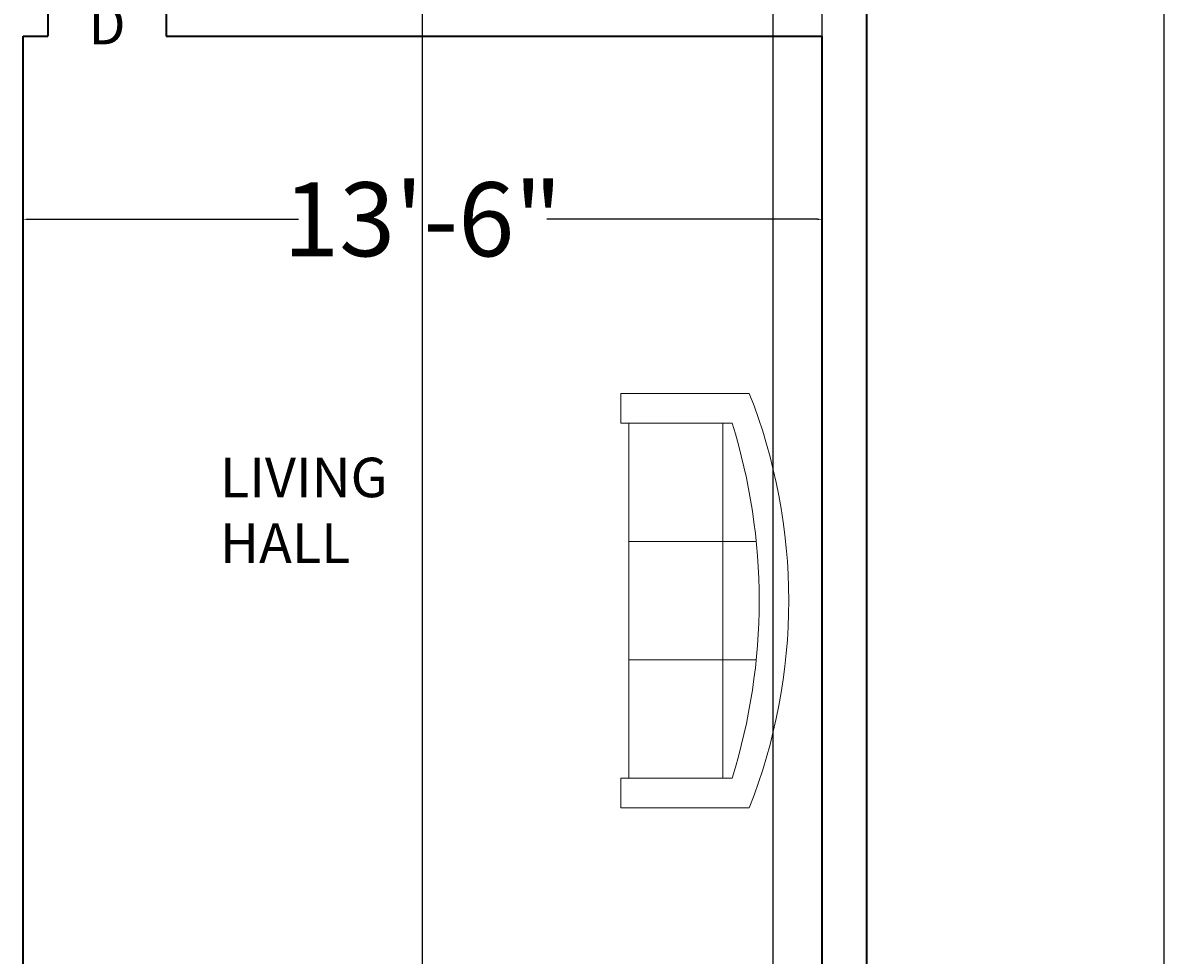
# Model space of a CAD drawing. Units: inches. Extents: x 371 to 1095, y -45 to 1219.
# Tile 13 of 18: x 862 to 1095, y 610 to 799. Entities that reach past the tile are written whole.
import ezdxf

# ---------------------------------------------------------------- set-up
doc = ezdxf.new("R2010")
doc.units = ezdxf.units.IN
doc.header["$MEASUREMENT"] = 0
for name, color, linetype, lineweight in [('A-ANNO-DIMS', 2, 'Continuous', 18), ('A-ANNO-TEXT', 7, 'Continuous', 18), ('A-AREA-IDEN', 7, 'Continuous', 18), ('A-FURN', 254, 'Continuous', 18), ('A-WALL', 40, 'Continuous', 35)]:
    doc.layers.add(name, color=color, linetype=linetype, lineweight=lineweight)
doc.styles.get("Standard").update_dxf_attribs({"font": 'arial.ttf'})
doc.dimstyles.get("Standard").update_dxf_attribs({"dimtxt": 1, "dimasz": 1, "dimexe": 0.18, "dimexo": 0.0625, "dimgap": 0.09, "dimtad": 0, "dimtih": 1, "dimtoh": 1, "dimdec": 0, "dimzin": 0, "dimdsep": 46, "dimlunit": 3, "dimtxsty": 'Standard', "dimcen": 0.09, "dimadec": 0, "dimazin": 0, "dimtfac": 1, "dimtdec": 0, "dimtofl": 0, "dimtmove": 0, "dimatfit": 3, "dimfxl": 1, "dimtolj": 1, "dimtzin": 0, "dimarcsym": 0})

# ---------------------------------------------------------------- blocks, each defined once
blk = doc.blocks.new('Sofa - Roundback 7 ft.')
for p, q in [((-12.00002, -32.4421), (-12.00003, -6.5971)), ((11.99997, -32.4421), (11.99998, -6.5971)), ((-36.000027, -34), (-36.000027, -11.4696)), ((35.99998, -34), (35.99998, -11.4696)), ((-35.999844, -13.3819), (35.9998, -13.3819)), ((-36.000027, -32.4421), (35.99998, -32.4421))]:
    blk.add_line(p, q)
for points in [[(-36.000027, -34), (-42.000027, -34), (-42.000027, -8)], [(41.99998, -8), (41.99998, -34), (35.99998, -34)]]:
    blk.add_lwpolyline(points)
for centre, radius, start, end in [((0, -114.25), 114.25, 68.43141, 111.5686), ((-0.00001, -127.1968), 121.1968, 72.72033, 107.2797)]:
    blk.add_arc(centre, radius, start, end)
blk = doc.blocks.new('*D24')
at = {"layer": 'A-ANNO-DIMS', "color": 0, "lineweight": -2, "transparency": 16777216}
for p, q in [((861.81, 748.67), (861.81, 759.09)), ((862.81, 758.91), (917.66, 758.91)), ((1022.81, 758.91), (967.96, 758.91)), ((1023.81, 748.67), (1023.81, 759.09))]:
    blk.add_line(p, q, dxfattribs=at)
at = {"layer": 'A-ANNO-DIMS', "color": 0, "transparency": 16777216}
for points in [[(862.81, 759.07), (862.81, 758.74), (861.81, 758.91)], [(1022.81, 759.07), (1022.81, 758.74), (1023.81, 758.91)]]:
    blk.add_solid(points, dxfattribs=at)
at = {"layer": 'Defpoints', "color": 0, "transparency": 16777216}
for p in [(1023.81, 758.91), (861.81, 748.61), (1023.81, 748.61)]:
    blk.add_point(p, dxfattribs=at)
at = {"layer": 'A-ANNO-DIMS', "color": 0, "transparency": 16777216, "insert": (942.81, 758.91), "char_height": 1, "attachment_point": 5}
blk.add_mtext('\\A1;{\\H15x;13\'-6"}', dxfattribs=at)
blk = doc.blocks.new('*D51')
at = {"layer": 'A-ANNO-DIMS', "color": 0, "lineweight": -2, "transparency": 16777216}
for p, q in [((1032.87, 982.03), (1093.19, 982.03)), ((1093.01, 981.03), (1093.01, 532.63)), ((1093.01, 83.03), (1093.01, 531.42)), ((1032.87, 82.03), (1093.19, 82.03))]:
    blk.add_line(p, q, dxfattribs=at)
at = {"layer": 'A-ANNO-DIMS', "color": 0, "transparency": 16777216}
for points in [[(1092.84, 981.03), (1093.17, 981.03), (1093.01, 982.03)], [(1092.84, 83.03), (1093.17, 83.03), (1093.01, 82.03)]]:
    blk.add_solid(points, dxfattribs=at)
at = {"layer": 'Defpoints', "color": 0, "transparency": 16777216}
for p in [(1032.81, 982.03), (1093.01, 982.03), (1032.81, 82.03)]:
    blk.add_point(p, dxfattribs=at)
at = {"layer": 'A-ANNO-DIMS', "color": 0, "transparency": 16777216, "insert": (1093.01, 532.03), "char_height": 1, "attachment_point": 5}
blk.add_mtext('\\A1;75\'-0"', dxfattribs=at)
blk = doc.blocks.new('*D63')
at = {"layer": 'A-ANNO-DIMS', "color": 0, "lineweight": -2, "transparency": 16777216}
for p, q in [((942.81, 580.09), (942.81, 1093.41)), ((943.81, 1093.23), (981.89, 1093.23)), ((1022.81, 1093.23), (984.73, 1093.23)), ((1023.81, 580.09), (1023.81, 1093.41))]:
    blk.add_line(p, q, dxfattribs=at)
at = {"layer": 'A-ANNO-DIMS', "color": 0, "transparency": 16777216}
for points in [[(943.81, 1093.39), (943.81, 1093.06), (942.81, 1093.23)], [(1022.81, 1093.39), (1022.81, 1093.06), (1023.81, 1093.23)]]:
    blk.add_solid(points, dxfattribs=at)
at = {"layer": 'Defpoints', "color": 0, "transparency": 16777216}
for p in [(1023.81, 1093.23), (942.81, 580.03), (1023.81, 580.03)]:
    blk.add_point(p, dxfattribs=at)
at = {"layer": 'A-ANNO-DIMS', "color": 0, "transparency": 16777216, "insert": (983.31, 1093.23), "char_height": 1, "attachment_point": 5}
blk.add_mtext('\\A1;6\'-9"', dxfattribs=at)
blk = doc.blocks.new('*D64')
at = {"layer": 'A-ANNO-DIMS', "color": 0, "lineweight": -2, "transparency": 16777216}
for p, q in [((1013.84, 464.01), (1013.84, 1093.41)), ((1014.84, 1093.23), (1017.01, 1093.23)), ((1022.81, 1093.23), (1020.63, 1093.23)), ((1023.81, 451.09), (1023.81, 1093.41))]:
    blk.add_line(p, q, dxfattribs=at)
at = {"layer": 'A-ANNO-DIMS', "color": 0, "transparency": 16777216}
for points in [[(1014.84, 1093.39), (1014.84, 1093.06), (1013.84, 1093.23)], [(1022.81, 1093.39), (1022.81, 1093.06), (1023.81, 1093.23)]]:
    blk.add_solid(points, dxfattribs=at)
at = {"layer": 'Defpoints', "color": 0, "transparency": 16777216}
for p in [(1023.81, 1093.23), (1013.84, 463.94), (1023.81, 451.03)]:
    blk.add_point(p, dxfattribs=at)
at = {"layer": 'A-ANNO-DIMS', "color": 0, "transparency": 16777216, "insert": (1018.82, 1093.23), "char_height": 1, "attachment_point": 5}
blk.add_mtext('\\A1;0\'-10"', dxfattribs=at)

msp = doc.modelspace()

# ---------------------------------------------------------------- linework, layer by layer
at = {"layer": 'A-WALL'}
for p, q in [((1032.81, 82.03), (1032.81, 982.03)), ((866.81, 805.03), (866.81, 796.03)), ((890.81, 805.03), (890.81, 796.03)), ((861.81, 796.03), (866.81, 796.03)), ((861.81, 451.03), (861.81, 796.03)), ((890.81, 796.03), (1023.81, 796.03)), ((1023.81, 580.03), (1023.81, 796.03))]:
    msp.add_line(p, q, dxfattribs=at)

# ---------------------------------------------------------------- block references
at = {"layer": 'A-FURN', "rotation": 270}
msp.add_blockref('Sofa - Roundback 7 ft.', (1017.01, 681.59), dxfattribs=at)

# ---------------------------------------------------------------- texts
at = {"layer": 'A-ANNO-TEXT', "insert": (875.09, 802.38), "char_height": 8, "attachment_point": 1}
msp.add_mtext_dynamic_manual_height_columns('D', width=17.4938, gutter_width=1, heights=[0], dxfattribs=at)
at = {"layer": 'A-AREA-IDEN', "insert": (901.72, 710.56), "char_height": 8, "attachment_point": 1}
msp.add_mtext_dynamic_manual_height_columns('LIVING HALL', width=53.6318, gutter_width=1, heights=[0], dxfattribs=at)

# ---------------------------------------------------------------- dimensions: what is measured, and where the dimension line sits
at = {"layer": 'A-ANNO-DIMS'}
for p1, p2, picture, middle in [((942.81, 580.03), (1023.81, 580.03), '*D63', (983.31, 1093.23)), ((1013.84, 463.94), (1023.81, 451.03), '*D64', (1018.82, 1093.23))]:
    dim = msp.add_linear_dim(base=(1023.81, 1093.23), p1=p1, p2=p2, dimstyle='Standard', override={"dimdec": 1, "dimlfac": 1, "dimrnd": 0, "dimzin": 1, "dimdsep": 46, "dimlunit": 4, "dimfrac": 2}, dxfattribs=at)
    dim.commit()
    dim.dimension.update_dxf_attribs({"geometry": picture, "text_midpoint": middle})
dim = msp.add_linear_dim(base=(1093.01, 982.03), p1=(1032.81, 82.03), p2=(1032.81, 982.03), angle=90, dimstyle='Standard', override={"dimdec": 1, "dimlfac": 1, "dimrnd": 0, "dimzin": 1, "dimdsep": 46, "dimlunit": 4, "dimfrac": 2}, dxfattribs=at)
dim.commit()
dim.dimension.update_dxf_attribs({"geometry": '*D51', "text_midpoint": (1093.01, 532.03)})
dim = msp.add_linear_dim(base=(1023.81, 758.91), p1=(861.81, 748.61), p2=(1023.81, 748.61), text='{\\H15x;<>}', dimstyle='Standard', override={"dimclrd": 0, "dimclre": 0, "dimclrt": 0}, dxfattribs=at)
dim.commit()
dim.dimension.update_dxf_attribs({"geometry": '*D24', "text_midpoint": (942.81, 758.91)})

doc.saveas('drawing.dxf')
